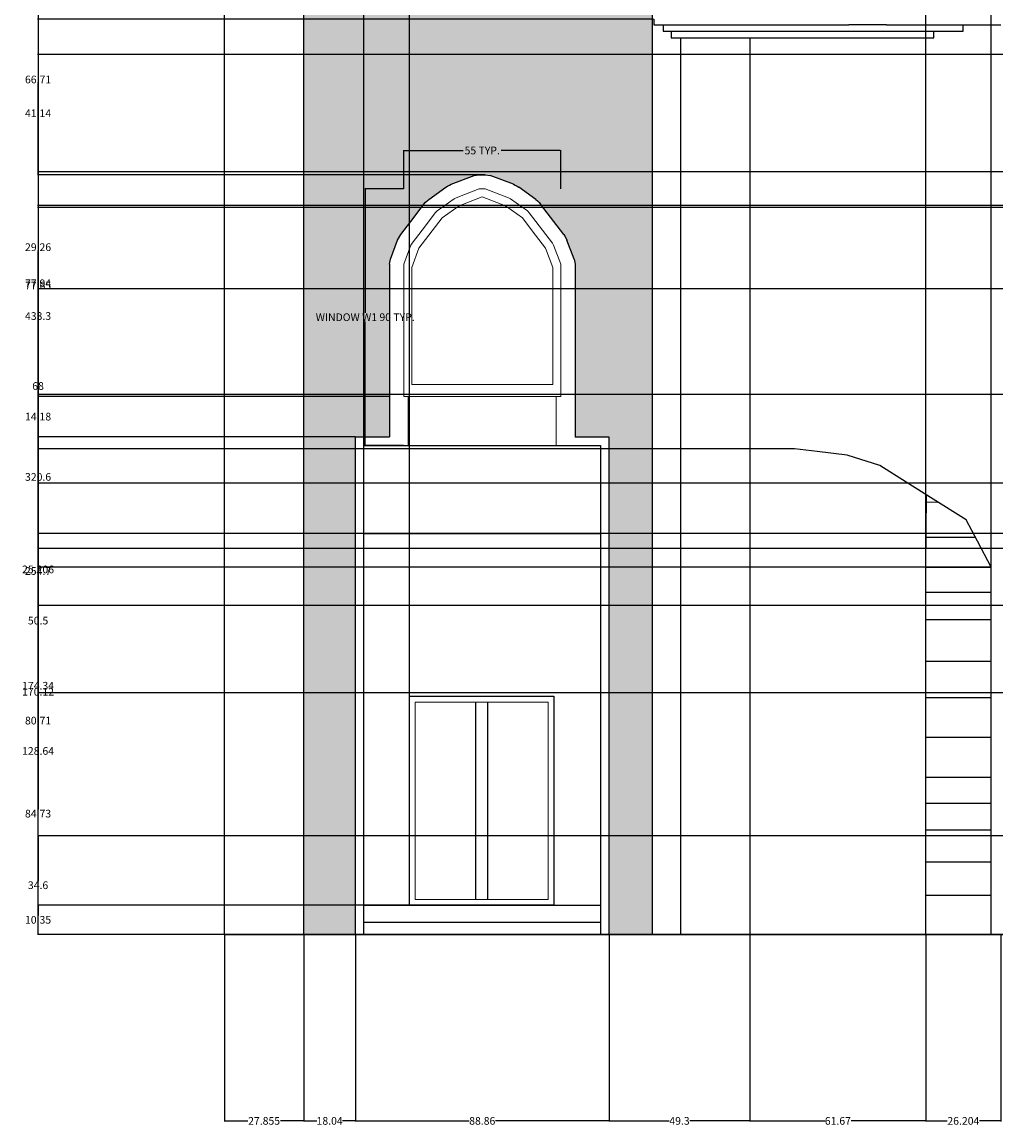
# Model space of a CAD drawing. Units: inches. Extents: x 2 to 1442, y 20 to 729.
# Tile 1 of 8: x 2 to 343, y 20 to 407. Entities that reach past the tile are written whole.
import ezdxf

# ---------------------------------------------------------------- set-up
doc = ezdxf.new("R2010")
doc.units = ezdxf.units.IN
doc.header["$MEASUREMENT"] = 0
for name, color, linetype, lineweight in [('A-ANNO-DIMS', 2, 'Continuous', 18), ('A-DOOR', 3, 'Continuous', 18), ('A-ELEV', 7, 'Continuous', 25), ('A-GLAZ', 4, 'Continuous', 18), ('A-WALL-PATT', 8, 'Continuous', 13)]:
    doc.layers.add(name, color=color, linetype=linetype, lineweight=lineweight)
doc.styles.get("Standard").update_dxf_attribs({"font": 'arial.ttf'})
doc.dimstyles.get("Standard").update_dxf_attribs({"dimtxt": 2.6875, "dimasz": 0.18, "dimexe": 0.18, "dimexo": 0.0625, "dimgap": 0.09, "dimtad": 0, "dimtih": 1, "dimtoh": 1, "dimdec": 4, "dimzin": 0, "dimdsep": 46, "dimlunit": 4, "dimtxsty": 'Standard', "dimcen": 0.09, "dimadec": 0, "dimazin": 0, "dimtfac": 1, "dimtdec": 4, "dimtofl": 0, "dimtmove": 0, "dimatfit": 3, "dimfxl": 1, "dimtolj": 1, "dimtzin": 0, "dimarcsym": 0})

# ---------------------------------------------------------------- blocks, each defined once
blk = doc.blocks.new('WIN-ARCH-TOWER')
for p, q in [((18.34, 86.78), (26.45, 89.83)), ((26.45, 89.83), (28.56, 89.83)), ((36.66, 86.78), (28.56, 89.83)), ((11.69, 82.12), (17.65, 86.41)), ((17.65, 86.41), (18.34, 86.78)), ((19.4, 83.98), (27.5, 87.02)), ((35.6, 83.98), (27.5, 87.02)), ((36.66, 86.78), (37.36, 86.41)), ((43.32, 82.12), (37.36, 86.41)), ((7.58, 76.95), (11.05, 81.5)), ((11.05, 81.5), (11.69, 82.12)), ((13.44, 79.69), (19.4, 83.98)), ((41.56, 79.69), (35.6, 83.98)), ((43.32, 82.12), (43.95, 81.5)), ((47.42, 76.95), (43.95, 81.5)), ((9.97, 75.13), (13.44, 79.69)), ((45.03, 75.13), (41.56, 79.69)), ((2.94, 70.87), (7.58, 76.95)), ((5.33, 69.05), (9.97, 75.13)), ((49.67, 69.05), (45.03, 75.13)), ((52.06, 70.87), (47.42, 76.95)), ((0, 63.44), (2.52, 70.11)), ((2.52, 70.11), (2.94, 70.87)), ((52.06, 70.87), (52.48, 70.11)), ((55, 63.44), (52.48, 70.11)), ((2.81, 62.38), (5.33, 69.05)), ((52.2, 62.38), (49.67, 69.05)), ((0, 63.44), (0, 62.38)), ((0, 62.38), (0, 17.18)), ((2.81, 21.32), (2.81, 62.38)), ((52.2, 21.32), (52.2, 62.38)), ((55, 63.44), (55, 62.38)), ((55, 62.38), (55, 17.41)), ((27.5, 21.32), (2.81, 21.32)), ((24.55, 21.32), (49.24, 21.32)), ((49.24, 21.32), (52.2, 21.32)), ((0, 17.18), (1.6, 17.18)), ((1.6, 0), (1.6, 17.18)), ((1.6, 17.18), (53.4, 17.18)), ((53.4, 0), (53.4, 17.18)), ((53.4, 17.18), (55.01, 17.18)), ((55.01, 17.18), (55, 17.41))]:
    blk.add_line(p, q)
blk = doc.blocks.new('DOOR-DOUBLE')
for points in [[(23.31, 0), (0, 0), (0, 69.12), (23.31, 69.12)], [(23.31, 69.12), (46.63, 69.12), (46.63, 0), (23.31, 0)]]:
    blk.add_lwpolyline(points)
blk = doc.blocks.new('*D5')
at = {"layer": 'A-ANNO-DIMS', "color": 0, "lineweight": -2, "transparency": 16777216}
for p, q in [((135.28, 348.44), (121.69, 348.44)), ((121.87, 348.26), (121.87, 305.01)), ((121.87, 258.79), (121.87, 302.05)), ((135.28, 258.61), (121.69, 258.61))]:
    blk.add_line(p, q, dxfattribs=at)
at = {"layer": 'A-ANNO-DIMS', "color": 0, "transparency": 16777216}
for points in [[(121.84, 348.26), (121.9, 348.26), (121.87, 348.44)], [(121.84, 258.79), (121.9, 258.79), (121.87, 258.61)]]:
    blk.add_solid(points, dxfattribs=at)
at = {"layer": 'Defpoints', "color": 0, "transparency": 16777216}
for p in [(121.87, 348.44), (135.35, 348.44), (135.35, 258.61)]:
    blk.add_point(p, dxfattribs=at)
at = {"layer": 'A-ANNO-DIMS', "color": 0, "transparency": 16777216, "insert": (121.87, 303.53), "char_height": 2.6875, "attachment_point": 5}
blk.add_mtext('\\A1;WINDOW W1 90 TYP.', dxfattribs=at)
blk = doc.blocks.new('*D6')
at = {"layer": 'A-ANNO-DIMS', "color": 0, "lineweight": -2, "transparency": 16777216}
for p, q in [((135.35, 348.5), (135.35, 362.09)), ((135.53, 361.91), (156.22, 361.91)), ((190.17, 361.91), (169.48, 361.91)), ((190.35, 348.5), (190.35, 362.09))]:
    blk.add_line(p, q, dxfattribs=at)
at = {"layer": 'A-ANNO-DIMS', "color": 0, "transparency": 16777216}
for points in [[(135.53, 361.94), (135.53, 361.88), (135.35, 361.91)], [(190.17, 361.94), (190.17, 361.88), (190.35, 361.91)]]:
    blk.add_solid(points, dxfattribs=at)
at = {"layer": 'Defpoints', "color": 0, "transparency": 16777216}
for p in [(190.35, 361.91), (135.35, 348.44), (190.35, 348.44)]:
    blk.add_point(p, dxfattribs=at)
at = {"layer": 'A-ANNO-DIMS', "color": 0, "transparency": 16777216, "insert": (162.85, 361.91), "char_height": 2.6875, "attachment_point": 5}
blk.add_mtext('\\A1;55 TYP.', dxfattribs=at)
blk = doc.blocks.new('*D13')
at = {"layer": 'A-ANNO-DIMS', "color": 0, "lineweight": -2, "transparency": 16777216}
for p, q in [((72.53, 87.21), (72.53, 21.84)), ((100.38, 87.21), (100.38, 21.84)), ((72.71, 22.02), (80.75, 22.02)), ((100.2, 22.02), (92.16, 22.02))]:
    blk.add_line(p, q, dxfattribs=at)
at = {"layer": 'A-ANNO-DIMS', "color": 0, "transparency": 16777216}
for points in [[(72.71, 22.05), (72.71, 21.99), (72.53, 22.02)], [(100.2, 22.05), (100.2, 21.99), (100.38, 22.02)]]:
    blk.add_solid(points, dxfattribs=at)
at = {"layer": 'Defpoints', "color": 0, "transparency": 16777216}
for p in [(72.53, 87.27), (100.38, 87.27), (100.38, 22.02)]:
    blk.add_point(p, dxfattribs=at)
at = {"layer": 'A-ANNO-DIMS', "color": 0, "transparency": 16777216, "insert": (86.45, 22.02), "char_height": 2.688, "attachment_point": 5}
blk.add_mtext('\\A1;27.855', dxfattribs=at)
blk = doc.blocks.new('*D14')
at = {"layer": 'A-ANNO-DIMS', "color": 0, "lineweight": -2, "transparency": 16777216}
for p, q in [((100.38, 87.21), (100.38, 21.84)), ((118.42, 87.21), (118.42, 21.84)), ((100.56, 22.02), (104.91, 22.02)), ((118.24, 22.02), (113.9, 22.02))]:
    blk.add_line(p, q, dxfattribs=at)
at = {"layer": 'A-ANNO-DIMS', "color": 0, "transparency": 16777216}
for points in [[(100.56, 22.05), (100.56, 21.99), (100.38, 22.02)], [(118.24, 22.05), (118.24, 21.99), (118.42, 22.02)]]:
    blk.add_solid(points, dxfattribs=at)
at = {"layer": 'Defpoints', "color": 0, "transparency": 16777216}
for p in [(100.38, 87.27), (118.42, 87.27), (118.42, 22.02)]:
    blk.add_point(p, dxfattribs=at)
at = {"layer": 'A-ANNO-DIMS', "color": 0, "transparency": 16777216, "insert": (109.4, 22.02), "char_height": 2.688, "attachment_point": 5}
blk.add_mtext('\\A1;18.04', dxfattribs=at)
blk = doc.blocks.new('*D15')
at = {"layer": 'A-ANNO-DIMS', "color": 0, "lineweight": -2, "transparency": 16777216}
for p, q in [((118.42, 87.21), (118.42, 21.84)), ((207.28, 87.21), (207.28, 21.84)), ((118.6, 22.02), (158.23, 22.02)), ((207.1, 22.02), (167.48, 22.02))]:
    blk.add_line(p, q, dxfattribs=at)
at = {"layer": 'A-ANNO-DIMS', "color": 0, "transparency": 16777216}
for points in [[(118.6, 22.05), (118.6, 21.99), (118.42, 22.02)], [(207.1, 22.05), (207.1, 21.99), (207.28, 22.02)]]:
    blk.add_solid(points, dxfattribs=at)
at = {"layer": 'Defpoints', "color": 0, "transparency": 16777216}
for p in [(118.42, 87.27), (207.28, 87.27), (207.28, 22.02)]:
    blk.add_point(p, dxfattribs=at)
at = {"layer": 'A-ANNO-DIMS', "color": 0, "transparency": 16777216, "insert": (162.85, 22.02), "char_height": 2.688, "attachment_point": 5}
blk.add_mtext('\\A1;88.86', dxfattribs=at)
blk = doc.blocks.new('*D16')
at = {"layer": 'A-ANNO-DIMS', "color": 0, "lineweight": -2, "transparency": 16777216}
for p, q in [((207.28, 87.21), (207.28, 21.84)), ((256.58, 87.21), (256.58, 21.84)), ((207.46, 22.02), (228.29, 22.02)), ((256.4, 22.02), (235.56, 22.02))]:
    blk.add_line(p, q, dxfattribs=at)
at = {"layer": 'A-ANNO-DIMS', "color": 0, "transparency": 16777216}
for points in [[(207.46, 22.05), (207.46, 21.99), (207.28, 22.02)], [(256.4, 22.05), (256.4, 21.99), (256.58, 22.02)]]:
    blk.add_solid(points, dxfattribs=at)
at = {"layer": 'Defpoints', "color": 0, "transparency": 16777216}
for p in [(207.28, 87.27), (256.58, 87.27), (256.58, 22.02)]:
    blk.add_point(p, dxfattribs=at)
at = {"layer": 'A-ANNO-DIMS', "color": 0, "transparency": 16777216, "insert": (231.93, 22.02), "char_height": 2.688, "attachment_point": 5}
blk.add_mtext('\\A1;49.3', dxfattribs=at)
blk = doc.blocks.new('*D17')
at = {"layer": 'A-ANNO-DIMS', "color": 0, "lineweight": -2, "transparency": 16777216}
for p, q in [((256.58, 87.21), (256.58, 21.84)), ((318.25, 87.21), (318.25, 21.84)), ((256.76, 22.02), (282.78, 22.02)), ((318.07, 22.02), (292.04, 22.02))]:
    blk.add_line(p, q, dxfattribs=at)
at = {"layer": 'A-ANNO-DIMS', "color": 0, "transparency": 16777216}
for points in [[(256.76, 22.05), (256.76, 21.99), (256.58, 22.02)], [(318.07, 22.05), (318.07, 21.99), (318.25, 22.02)]]:
    blk.add_solid(points, dxfattribs=at)
at = {"layer": 'Defpoints', "color": 0, "transparency": 16777216}
for p in [(256.58, 87.27), (318.25, 87.27), (318.25, 22.02)]:
    blk.add_point(p, dxfattribs=at)
at = {"layer": 'A-ANNO-DIMS', "color": 0, "transparency": 16777216, "insert": (287.41, 22.02), "char_height": 2.688, "attachment_point": 5}
blk.add_mtext('\\A1;61.67', dxfattribs=at)
blk = doc.blocks.new('*D18')
at = {"layer": 'A-ANNO-DIMS', "color": 0, "lineweight": -2, "transparency": 16777216}
for p, q in [((318.25, 87.21), (318.25, 21.84)), ((344.45, 87.21), (344.45, 21.84)), ((318.43, 22.02), (325.66, 22.02)), ((344.27, 22.02), (337.04, 22.02))]:
    blk.add_line(p, q, dxfattribs=at)
at = {"layer": 'A-ANNO-DIMS', "color": 0, "transparency": 16777216}
for points in [[(318.43, 22.05), (318.43, 21.99), (318.25, 22.02)], [(344.27, 22.05), (344.27, 21.99), (344.45, 22.02)]]:
    blk.add_solid(points, dxfattribs=at)
at = {"layer": 'Defpoints', "color": 0, "transparency": 16777216}
for p in [(318.25, 87.27), (344.45, 87.27), (344.45, 22.02)]:
    blk.add_point(p, dxfattribs=at)
at = {"layer": 'A-ANNO-DIMS', "color": 0, "transparency": 16777216, "insert": (331.35, 22.02), "char_height": 2.688, "attachment_point": 5}
blk.add_mtext('\\A1;26.204', dxfattribs=at)
blk = doc.blocks.new('*D32')
at = {"layer": 'A-ANNO-DIMS', "color": 0, "lineweight": -2, "transparency": 16777216}
for p, q in [((72.46, 520.58), (7.1, 520.58)), ((7.28, 520.4), (7.28, 305.39)), ((7.28, 87.45), (7.28, 302.46)), ((72.46, 87.27), (7.1, 87.27))]:
    blk.add_line(p, q, dxfattribs=at)
at = {"layer": 'A-ANNO-DIMS', "color": 0, "transparency": 16777216}
for points in [[(7.25, 520.4), (7.31, 520.4), (7.28, 520.58)], [(7.25, 87.45), (7.31, 87.45), (7.28, 87.27)]]:
    blk.add_solid(points, dxfattribs=at)
at = {"layer": 'Defpoints', "color": 0, "transparency": 16777216}
for p in [(7.28, 520.58), (72.53, 520.58), (72.53, 87.27)]:
    blk.add_point(p, dxfattribs=at)
at = {"layer": 'A-ANNO-DIMS', "color": 0, "transparency": 16777216, "insert": (7.28, 303.93), "char_height": 2.688, "attachment_point": 5}
blk.add_mtext('\\A1;433.3', dxfattribs=at)
blk = doc.blocks.new('*D34')
at = {"layer": 'A-ANNO-DIMS', "color": 0, "lineweight": -2, "transparency": 16777216}
for p, q in [((118.36, 261.61), (7.1, 261.61)), ((7.28, 261.43), (7.28, 175.9)), ((7.28, 87.45), (7.28, 172.98)), ((100.32, 87.27), (7.1, 87.27))]:
    blk.add_line(p, q, dxfattribs=at)
at = {"layer": 'A-ANNO-DIMS', "color": 0, "transparency": 16777216}
for points in [[(7.25, 261.43), (7.31, 261.43), (7.28, 261.61)], [(7.25, 87.45), (7.31, 87.45), (7.28, 87.27)]]:
    blk.add_solid(points, dxfattribs=at)
at = {"layer": 'Defpoints', "color": 0, "transparency": 16777216}
for p in [(118.42, 261.61), (7.28, 87.27), (100.38, 87.27)]:
    blk.add_point(p, dxfattribs=at)
at = {"layer": 'A-ANNO-DIMS', "color": 0, "transparency": 16777216, "insert": (7.28, 174.44), "char_height": 2.688, "attachment_point": 5}
blk.add_mtext('\\A1;174.34', dxfattribs=at)
blk = doc.blocks.new('*D35')
at = {"layer": 'A-ANNO-DIMS', "color": 0, "lineweight": -2, "transparency": 16777216}
for p, q in [((130.28, 275.79), (7.1, 275.79)), ((7.28, 275.61), (7.28, 270.16)), ((7.28, 261.79), (7.28, 267.24)), ((118.36, 261.61), (7.1, 261.61))]:
    blk.add_line(p, q, dxfattribs=at)
at = {"layer": 'A-ANNO-DIMS', "color": 0, "transparency": 16777216}
for points in [[(7.25, 275.61), (7.31, 275.61), (7.28, 275.79)], [(7.25, 261.79), (7.31, 261.79), (7.28, 261.61)]]:
    blk.add_solid(points, dxfattribs=at)
at = {"layer": 'Defpoints', "color": 0, "transparency": 16777216}
for p in [(7.28, 275.79), (130.35, 275.79), (118.42, 261.61)]:
    blk.add_point(p, dxfattribs=at)
at = {"layer": 'A-ANNO-DIMS', "color": 0, "transparency": 16777216, "insert": (7.28, 268.7), "char_height": 2.688, "attachment_point": 5}
blk.add_mtext('\\A1;14.18', dxfattribs=at)
blk = doc.blocks.new('*D36')
at = {"layer": 'A-ANNO-DIMS', "color": 0, "lineweight": -2, "transparency": 16777216}
for p, q in [((163.84, 353.44), (7.1, 353.44)), ((7.28, 353.26), (7.28, 316.08)), ((7.28, 275.97), (7.28, 313.15)), ((130.28, 275.79), (7.1, 275.79))]:
    blk.add_line(p, q, dxfattribs=at)
at = {"layer": 'A-ANNO-DIMS', "color": 0, "transparency": 16777216}
for points in [[(7.25, 353.26), (7.31, 353.26), (7.28, 353.44)], [(7.25, 275.97), (7.31, 275.97), (7.28, 275.79)]]:
    blk.add_solid(points, dxfattribs=at)
at = {"layer": 'Defpoints', "color": 0, "transparency": 16777216}
for p in [(7.28, 353.44), (163.9, 353.44), (130.35, 275.79)]:
    blk.add_point(p, dxfattribs=at)
at = {"layer": 'A-ANNO-DIMS', "color": 0, "transparency": 16777216, "insert": (7.28, 314.62), "char_height": 2.688, "attachment_point": 5}
blk.add_mtext('\\A1;77.65', dxfattribs=at)
blk = doc.blocks.new('*D37')
at = {"layer": 'A-ANNO-DIMS', "color": 0, "lineweight": -2, "transparency": 16777216}
for p, q in [((144.79, 420.15), (7.1, 420.15)), ((7.28, 419.97), (7.28, 388.26)), ((7.28, 353.62), (7.28, 385.33)), ((163.84, 353.44), (7.1, 353.44))]:
    blk.add_line(p, q, dxfattribs=at)
at = {"layer": 'A-ANNO-DIMS', "color": 0, "transparency": 16777216}
for points in [[(7.25, 419.97), (7.31, 419.97), (7.28, 420.15)], [(7.25, 353.62), (7.31, 353.62), (7.28, 353.44)]]:
    blk.add_solid(points, dxfattribs=at)
at = {"layer": 'Defpoints', "color": 0, "transparency": 16777216}
for p in [(7.28, 420.15), (144.86, 420.15), (163.9, 353.44)]:
    blk.add_point(p, dxfattribs=at)
at = {"layer": 'A-ANNO-DIMS', "color": 0, "transparency": 16777216, "insert": (7.28, 386.79), "char_height": 2.688, "attachment_point": 5}
blk.add_mtext('\\A1;66.71', dxfattribs=at)
blk = doc.blocks.new('*D41')
at = {"layer": 'A-ANNO-DIMS', "color": 0, "lineweight": -2, "transparency": 16777216}
for p, q in [((137.28, 97.62), (7.1, 97.62)), ((7.28, 97.44), (7.28, 93.91)), ((7.28, 87.45), (7.28, 90.98)), ((121.36, 87.27), (7.1, 87.27))]:
    blk.add_line(p, q, dxfattribs=at)
at = {"layer": 'A-ANNO-DIMS', "color": 0, "transparency": 16777216}
for points in [[(7.25, 97.44), (7.31, 97.44), (7.28, 97.62)], [(7.25, 87.45), (7.31, 87.45), (7.28, 87.27)]]:
    blk.add_solid(points, dxfattribs=at)
at = {"layer": 'Defpoints', "color": 0, "transparency": 16777216}
for p in [(137.34, 97.62), (7.28, 87.27), (121.42, 87.27)]:
    blk.add_point(p, dxfattribs=at)
at = {"layer": 'A-ANNO-DIMS', "color": 0, "transparency": 16777216, "insert": (7.28, 92.45), "char_height": 2.688, "attachment_point": 5}
blk.add_mtext('\\A1;10.35', dxfattribs=at)
blk = doc.blocks.new('*D42')
at = {"layer": 'A-ANNO-DIMS', "color": 0, "lineweight": -2, "transparency": 16777216}
for p, q in [((121.42, 97.68), (121.42, 726.93)), ((137.34, 97.68), (137.34, 726.93)), ((121.6, 726.75), (123.84, 726.75)), ((137.16, 726.75), (134.93, 726.75))]:
    blk.add_line(p, q, dxfattribs=at)
at = {"layer": 'A-ANNO-DIMS', "color": 0, "transparency": 16777216}
for points in [[(121.6, 726.78), (121.6, 726.72), (121.42, 726.75)], [(137.16, 726.78), (137.16, 726.72), (137.34, 726.75)]]:
    blk.add_solid(points, dxfattribs=at)
at = {"layer": 'Defpoints', "color": 0, "transparency": 16777216}
for p in [(137.34, 726.75), (121.42, 97.62), (137.34, 97.62)]:
    blk.add_point(p, dxfattribs=at)
at = {"layer": 'A-ANNO-DIMS', "color": 0, "transparency": 16777216, "insert": (129.38, 726.75), "char_height": 2.688, "attachment_point": 5}
blk.add_mtext('\\A1;15.918', dxfattribs=at)
blk = doc.blocks.new('*D43')
at = {"layer": 'A-ANNO-DIMS', "color": 0, "lineweight": -2, "transparency": 16777216}
for p, q in [((222.84, 407.89), (7.1, 407.89)), ((7.28, 407.71), (7.28, 249.04)), ((7.28, 87.45), (7.28, 246.12)), ((232.22, 87.27), (7.1, 87.27))]:
    blk.add_line(p, q, dxfattribs=at)
at = {"layer": 'A-ANNO-DIMS', "color": 0, "transparency": 16777216}
for points in [[(7.25, 407.71), (7.31, 407.71), (7.28, 407.89)], [(7.25, 87.45), (7.31, 87.45), (7.28, 87.27)]]:
    blk.add_solid(points, dxfattribs=at)
at = {"layer": 'Defpoints', "color": 0, "transparency": 16777216}
for p in [(7.28, 407.89), (222.9, 407.89), (232.28, 87.27)]:
    blk.add_point(p, dxfattribs=at)
at = {"layer": 'A-ANNO-DIMS', "color": 0, "transparency": 16777216, "insert": (7.28, 247.58), "char_height": 2.688, "attachment_point": 5}
blk.add_mtext('\\A1;320.6', dxfattribs=at)
blk = doc.blocks.new('*D46')
at = {"layer": 'A-ANNO-DIMS', "color": 0, "lineweight": -2, "transparency": 16777216}
for p, q in [((341, 215.92), (7.1, 215.92)), ((7.28, 215.74), (7.28, 153.06)), ((7.28, 87.45), (7.28, 150.13)), ((318.18, 87.27), (7.1, 87.27))]:
    blk.add_line(p, q, dxfattribs=at)
at = {"layer": 'A-ANNO-DIMS', "color": 0, "transparency": 16777216}
for points in [[(7.25, 215.74), (7.31, 215.74), (7.28, 215.92)], [(7.25, 87.45), (7.31, 87.45), (7.28, 87.27)]]:
    blk.add_solid(points, dxfattribs=at)
at = {"layer": 'Defpoints', "color": 0, "transparency": 16777216}
for p in [(7.28, 215.92), (341.06, 215.92), (318.25, 87.27)]:
    blk.add_point(p, dxfattribs=at)
at = {"layer": 'A-ANNO-DIMS', "color": 0, "transparency": 16777216, "insert": (7.28, 151.59), "char_height": 2.688, "attachment_point": 5}
blk.add_mtext('\\A1;128.64', dxfattribs=at)
blk = doc.blocks.new('*D47')
at = {"layer": 'A-ANNO-DIMS', "color": 0, "lineweight": -2, "transparency": 16777216}
for p, q in [((318.25, 215.98), (318.25, 726.93)), ((341.06, 215.98), (341.06, 726.93)), ((318.43, 726.75), (323.95, 726.75)), ((340.88, 726.75), (335.36, 726.75))]:
    blk.add_line(p, q, dxfattribs=at)
at = {"layer": 'A-ANNO-DIMS', "color": 0, "transparency": 16777216}
for points in [[(318.43, 726.78), (318.43, 726.72), (318.25, 726.75)], [(340.88, 726.78), (340.88, 726.72), (341.06, 726.75)]]:
    blk.add_solid(points, dxfattribs=at)
at = {"layer": 'Defpoints', "color": 0, "transparency": 16777216}
for p in [(341.06, 726.75), (318.25, 215.92), (341.06, 215.92)]:
    blk.add_point(p, dxfattribs=at)
at = {"layer": 'A-ANNO-DIMS', "color": 0, "transparency": 16777216, "insert": (329.65, 726.75), "char_height": 2.688, "attachment_point": 5}
blk.add_mtext('\\A1;22.815', dxfattribs=at)
blk = doc.blocks.new('*D48')
at = {"layer": 'A-ANNO-DIMS', "color": 0, "lineweight": -2, "transparency": 16777216}
for p, q in [((256.51, 257.39), (7.1, 257.39)), ((7.28, 257.21), (7.28, 173.79)), ((7.28, 87.45), (7.28, 170.87)), ((256.51, 87.27), (7.1, 87.27))]:
    blk.add_line(p, q, dxfattribs=at)
at = {"layer": 'A-ANNO-DIMS', "color": 0, "transparency": 16777216}
for points in [[(7.25, 257.21), (7.31, 257.21), (7.28, 257.39)], [(7.25, 87.45), (7.31, 87.45), (7.28, 87.27)]]:
    blk.add_solid(points, dxfattribs=at)
at = {"layer": 'Defpoints', "color": 0, "transparency": 16777216}
for p in [(256.58, 257.39), (7.28, 87.27), (256.58, 87.27)]:
    blk.add_point(p, dxfattribs=at)
at = {"layer": 'A-ANNO-DIMS', "color": 0, "transparency": 16777216, "insert": (7.28, 172.33), "char_height": 2.688, "attachment_point": 5}
blk.add_mtext('\\A1;170.12', dxfattribs=at)
blk = doc.blocks.new('*D54')
at = {"layer": 'A-ANNO-DIMS', "color": 0, "lineweight": -2, "transparency": 16777216}
for p, q in [((388.65, 354.39), (7.1, 354.39)), ((7.28, 354.21), (7.28, 316.88)), ((7.28, 276.62), (7.28, 313.95)), ((353.03, 276.44), (7.1, 276.44))]:
    blk.add_line(p, q, dxfattribs=at)
at = {"layer": 'A-ANNO-DIMS', "color": 0, "transparency": 16777216}
for points in [[(7.25, 354.21), (7.31, 354.21), (7.28, 354.39)], [(7.25, 276.62), (7.31, 276.62), (7.28, 276.44)]]:
    blk.add_solid(points, dxfattribs=at)
at = {"layer": 'Defpoints', "color": 0, "transparency": 16777216}
for p in [(7.28, 354.39), (388.71, 354.39), (353.09, 276.44)]:
    blk.add_point(p, dxfattribs=at)
at = {"layer": 'A-ANNO-DIMS', "color": 0, "transparency": 16777216, "insert": (7.28, 315.41), "char_height": 2.688, "attachment_point": 5}
blk.add_mtext('\\A1;77.94', dxfattribs=at)
blk = doc.blocks.new('*D57')
at = {"layer": 'A-ANNO-DIMS', "color": 0, "lineweight": -2, "transparency": 16777216}
for p, q in [((381.96, 395.53), (7.1, 395.53)), ((7.28, 395.35), (7.28, 376.4)), ((7.28, 354.57), (7.28, 373.52)), ((388.65, 354.39), (7.1, 354.39))]:
    blk.add_line(p, q, dxfattribs=at)
at = {"layer": 'A-ANNO-DIMS', "color": 0, "transparency": 16777216}
for points in [[(7.25, 395.35), (7.31, 395.35), (7.28, 395.53)], [(7.25, 354.57), (7.31, 354.57), (7.28, 354.39)]]:
    blk.add_solid(points, dxfattribs=at)
at = {"layer": 'Defpoints', "color": 0, "transparency": 16777216}
for p in [(382.02, 395.53), (7.28, 354.39), (388.71, 354.39)]:
    blk.add_point(p, dxfattribs=at)
at = {"layer": 'A-ANNO-DIMS', "color": 0, "transparency": 16777216, "insert": (7.28, 374.96), "char_height": 2.688, "attachment_point": 5}
blk.add_mtext('\\A1;41.14', dxfattribs=at)
blk = doc.blocks.new('*D72')
at = {"layer": 'A-ANNO-DIMS', "color": 0, "lineweight": -2, "transparency": 16777216}
for p, q in [((585.94, 341.99), (7.1, 341.99)), ((7.28, 341.81), (7.28, 216.09)), ((7.28, 87.45), (7.28, 213.17)), ((592.44, 87.27), (7.1, 87.27))]:
    blk.add_line(p, q, dxfattribs=at)
at = {"layer": 'A-ANNO-DIMS', "color": 0, "transparency": 16777216}
for points in [[(7.25, 341.81), (7.31, 341.81), (7.28, 341.99)], [(7.25, 87.45), (7.31, 87.45), (7.28, 87.27)]]:
    blk.add_solid(points, dxfattribs=at)
at = {"layer": 'Defpoints', "color": 0, "transparency": 16777216}
for p in [(7.28, 341.99), (586, 341.99), (592.5, 87.27)]:
    blk.add_point(p, dxfattribs=at)
at = {"layer": 'A-ANNO-DIMS', "color": 0, "transparency": 16777216, "insert": (7.28, 214.63), "char_height": 2.688, "attachment_point": 5}
blk.add_mtext('\\A1;254.7', dxfattribs=at)
blk = doc.blocks.new('*D74')
at = {"layer": 'A-ANNO-DIMS', "color": 0, "lineweight": -2, "transparency": 16777216}
for p, q in [((655.94, 172), (7.1, 172)), ((7.28, 171.82), (7.28, 131.1)), ((7.28, 87.45), (7.28, 128.17)), ((655.94, 87.27), (7.1, 87.27))]:
    blk.add_line(p, q, dxfattribs=at)
at = {"layer": 'A-ANNO-DIMS', "color": 0, "transparency": 16777216}
for points in [[(7.25, 171.82), (7.31, 171.82), (7.28, 172)], [(7.25, 87.45), (7.31, 87.45), (7.28, 87.27)]]:
    blk.add_solid(points, dxfattribs=at)
at = {"layer": 'Defpoints', "color": 0, "transparency": 16777216}
for p in [(656, 172), (7.28, 87.27), (656, 87.27)]:
    blk.add_point(p, dxfattribs=at)
at = {"layer": 'A-ANNO-DIMS', "color": 0, "transparency": 16777216, "insert": (7.28, 129.64), "char_height": 2.688, "attachment_point": 5}
blk.add_mtext('\\A1;84.73', dxfattribs=at)
blk = doc.blocks.new('*D75')
at = {"layer": 'A-ANNO-DIMS', "color": 0, "lineweight": -2, "transparency": 16777216}
for p, q in [((721.76, 222.5), (7.1, 222.5)), ((7.28, 222.32), (7.28, 198.71)), ((7.28, 172.18), (7.28, 195.79)), ((655.94, 172), (7.1, 172))]:
    blk.add_line(p, q, dxfattribs=at)
at = {"layer": 'A-ANNO-DIMS', "color": 0, "transparency": 16777216}
for points in [[(7.25, 222.32), (7.31, 222.32), (7.28, 222.5)], [(7.25, 172.18), (7.31, 172.18), (7.28, 172)]]:
    blk.add_solid(points, dxfattribs=at)
at = {"layer": 'Defpoints', "color": 0, "transparency": 16777216}
for p in [(7.28, 222.5), (721.83, 222.5), (656, 172)]:
    blk.add_point(p, dxfattribs=at)
at = {"layer": 'A-ANNO-DIMS', "color": 0, "transparency": 16777216, "insert": (7.28, 197.25), "char_height": 2.688, "attachment_point": 5}
blk.add_mtext('\\A1;50.5', dxfattribs=at)
blk = doc.blocks.new('*D76')
at = {"layer": 'A-ANNO-DIMS', "color": 0, "lineweight": -2, "transparency": 16777216}
for p, q in [((470.75, 121.87), (7.1, 121.87)), ((7.28, 121.69), (7.28, 106.03)), ((7.28, 87.45), (7.28, 103.11)), ((470.75, 87.27), (7.1, 87.27))]:
    blk.add_line(p, q, dxfattribs=at)
at = {"layer": 'A-ANNO-DIMS', "color": 0, "transparency": 16777216}
for points in [[(7.25, 121.69), (7.31, 121.69), (7.28, 121.87)], [(7.25, 87.45), (7.31, 87.45), (7.28, 87.27)]]:
    blk.add_solid(points, dxfattribs=at)
at = {"layer": 'Defpoints', "color": 0, "transparency": 16777216}
for p in [(470.81, 121.87), (7.28, 87.27), (470.81, 87.27)]:
    blk.add_point(p, dxfattribs=at)
at = {"layer": 'A-ANNO-DIMS', "color": 0, "transparency": 16777216, "insert": (7.28, 104.57), "char_height": 2.688, "attachment_point": 5}
blk.add_mtext('\\A1;34.6', dxfattribs=at)
blk = doc.blocks.new('*D77')
at = {"layer": 'A-ANNO-DIMS', "color": 0, "lineweight": -2, "transparency": 16777216}
for p, q in [((470.75, 202.58), (7.1, 202.58)), ((7.28, 202.4), (7.28, 163.69)), ((7.28, 122.05), (7.28, 160.77)), ((470.75, 121.87), (7.1, 121.87))]:
    blk.add_line(p, q, dxfattribs=at)
at = {"layer": 'A-ANNO-DIMS', "color": 0, "transparency": 16777216}
for points in [[(7.25, 202.4), (7.31, 202.4), (7.28, 202.58)], [(7.25, 122.05), (7.31, 122.05), (7.28, 121.87)]]:
    blk.add_solid(points, dxfattribs=at)
at = {"layer": 'Defpoints', "color": 0, "transparency": 16777216}
for p in [(7.28, 202.58), (470.81, 202.58), (470.81, 121.87)]:
    blk.add_point(p, dxfattribs=at)
at = {"layer": 'A-ANNO-DIMS', "color": 0, "transparency": 16777216, "insert": (7.28, 162.23), "char_height": 2.688, "attachment_point": 5}
blk.add_mtext('\\A1;80.71', dxfattribs=at)
blk = doc.blocks.new('*D78')
at = {"layer": 'A-ANNO-DIMS', "color": 0, "lineweight": -2, "transparency": 16777216}
for p, q in [((470.75, 227.79), (7.1, 227.79)), ((7.28, 227.61), (7.28, 216.65)), ((7.28, 202.76), (7.28, 213.72)), ((470.75, 202.58), (7.1, 202.58))]:
    blk.add_line(p, q, dxfattribs=at)
at = {"layer": 'A-ANNO-DIMS', "color": 0, "transparency": 16777216}
for points in [[(7.25, 227.61), (7.31, 227.61), (7.28, 227.79)], [(7.25, 202.76), (7.31, 202.76), (7.28, 202.58)]]:
    blk.add_solid(points, dxfattribs=at)
at = {"layer": 'Defpoints', "color": 0, "transparency": 16777216}
for p in [(7.28, 227.79), (470.81, 227.79), (470.81, 202.58)]:
    blk.add_point(p, dxfattribs=at)
at = {"layer": 'A-ANNO-DIMS', "color": 0, "transparency": 16777216, "insert": (7.28, 215.19), "char_height": 2.688, "attachment_point": 5}
blk.add_mtext('\\A1;25.206', dxfattribs=at)
blk = doc.blocks.new('*D79')
at = {"layer": 'A-ANNO-DIMS', "color": 0, "lineweight": -2, "transparency": 16777216}
for p, q in [((489.71, 313.43), (7.1, 313.43)), ((7.28, 313.25), (7.28, 280.88)), ((7.28, 245.6), (7.28, 277.96)), ((489.71, 245.42), (7.1, 245.42))]:
    blk.add_line(p, q, dxfattribs=at)
at = {"layer": 'A-ANNO-DIMS', "color": 0, "transparency": 16777216}
for points in [[(7.25, 313.25), (7.31, 313.25), (7.28, 313.43)], [(7.25, 245.6), (7.31, 245.6), (7.28, 245.42)]]:
    blk.add_solid(points, dxfattribs=at)
at = {"layer": 'Defpoints', "color": 0, "transparency": 16777216}
for p in [(7.28, 313.43), (489.77, 313.43), (489.77, 245.42)]:
    blk.add_point(p, dxfattribs=at)
at = {"layer": 'A-ANNO-DIMS', "color": 0, "transparency": 16777216, "insert": (7.28, 279.42), "char_height": 2.688, "attachment_point": 5}
blk.add_mtext('\\A1;68', dxfattribs=at)
blk = doc.blocks.new('*D80')
at = {"layer": 'A-ANNO-DIMS', "color": 0, "lineweight": -2, "transparency": 16777216}
for p, q in [((526.66, 342.68), (7.1, 342.68)), ((7.28, 342.5), (7.28, 329.52)), ((7.28, 313.61), (7.28, 326.59)), ((489.71, 313.43), (7.1, 313.43))]:
    blk.add_line(p, q, dxfattribs=at)
at = {"layer": 'A-ANNO-DIMS', "color": 0, "transparency": 16777216}
for points in [[(7.25, 342.5), (7.31, 342.5), (7.28, 342.68)], [(7.25, 313.61), (7.31, 313.61), (7.28, 313.43)]]:
    blk.add_solid(points, dxfattribs=at)
at = {"layer": 'Defpoints', "color": 0, "transparency": 16777216}
for p in [(7.28, 342.68), (526.72, 342.68), (489.77, 313.43)]:
    blk.add_point(p, dxfattribs=at)
at = {"layer": 'A-ANNO-DIMS', "color": 0, "transparency": 16777216, "insert": (7.28, 328.05), "char_height": 2.688, "attachment_point": 5}
blk.add_mtext('\\A1;29.26', dxfattribs=at)

msp = doc.modelspace()

# ---------------------------------------------------------------- hatches: boundary and pattern name
at = {"layer": 'A-WALL-PATT'}
h = msp.add_hatch(dxfattribs=at)
h.set_pattern_fill('BRASS', color=256, scale=14)
h.paths.add_polyline_path([(222.3553, 494.0357), (100.382, 494.0357), (100.382, 87.2714), (118.4234, 87.2714), (118.4234, 261.6116), (130.3451, 261.6116), (130.3451, 275.7919), (130.3451, 320.992), (130.3451, 322.0535), (130.6686, 323.8227), (133.191, 330.4901), (134.3119, 332.5101), (138.9535, 338.5974), (142.6478, 343.4423), (143.8105, 344.5736), (150.3377, 349.2734), (151.6201, 349.9601), (160.0334, 353.1203), (161.7915, 353.4396), (163.9013, 353.4396), (165.6594, 353.1203), (174.0727, 349.9601), (175.3551, 349.2734), (181.8823, 344.5736), (183.045, 343.4423), (186.7393, 338.5974), (191.601, 332.2216), (192.3734, 330.8295), (195.0242, 323.8227), (195.3477, 322.0535), (195.3477, 320.992), (195.3477, 276.0187), (195.3477, 261.5562), (207.2798, 261.5562), (207.2798, 87.2714), (222.3553, 87.2714)])
h.paths.add_polyline_path([(144.8571, 420.1495), (144.8571, 464.3282), (148.784, 472.9254), (157.7288, 481.8631), (164.2287, 486.0178), (170.7285, 481.8631), (179.6733, 472.9254), (183.6002, 464.3282), (183.6002, 420.1495)], flags=16)
h.paths.add_polyline_path([(146.8571, 422.1495), (146.8571, 463.893), (150.4531, 471.7659), (158.9889, 480.2948), (164.2287, 483.6441), (169.4684, 480.2948), (178.0042, 471.7659), (181.6002, 463.893), (181.6002, 422.1495)], flags=0)

# ---------------------------------------------------------------- linework, layer by layer
at = {"layer": 'A-ELEV'}
for p, q in [((72.5272, 255.2714), (72.5272, 423.2714)), ((222.8994, 407.8873), (222.8994, 405.9114)), ((222.8994, 405.9114), (249.3478, 405.9114)), ((226.1729, 405.9114), (226.1729, 403.6578)), ((226.1729, 403.6578), (249.3478, 403.6578)), ((229.0144, 403.6578), (229.0144, 401.3516)), ((249.3478, 405.9114), (291.2886, 405.9114)), ((249.3478, 403.6578), (299.4874, 403.6578)), ((304.4461, 405.9114), (291.2886, 405.9114)), ((299.4874, 403.6578), (331.3076, 403.6578)), ((304.4461, 405.9114), (335.8829, 405.9114)), ((321.0095, 401.3516), (321.0095, 403.6578)), ((331.3076, 403.6578), (331.3076, 405.9114)), ((335.8829, 405.9114), (335.8829, 405.9114)), ((335.8829, 405.9114), (344.4513, 405.9114)), ((229.0144, 401.3516), (291.0961, 401.3516)), ((232.2824, 401.3516), (232.2824, 87.2714)), ((256.5766, 401.3516), (256.5766, 87.2714)), ((291.0961, 401.3516), (321.0095, 401.3516)), ((151.9303, 350.0767), (160.0334, 353.1203)), ((161.7915, 353.4396), (163.9013, 353.4396)), ((173.7625, 350.0767), (165.6594, 353.1203)), ((144.1106, 344.7897), (150.0687, 349.0797)), ((150.6298, 349.4298), (151.3279, 349.8037)), ((174.3649, 349.8037), (175.063, 349.4298)), ((181.5822, 344.7897), (175.6241, 349.0797)), ((142.9129, 343.7002), (143.5455, 344.3157)), ((182.1473, 344.3157), (182.7799, 343.7002)), ((138.9535, 338.5974), (142.4236, 343.1483)), ((186.7393, 338.5974), (183.2692, 343.1483)), ((134.3119, 332.5101), (138.9535, 338.5974)), ((191.381, 332.5101), (186.7393, 338.5974)), ((130.6686, 323.8227), (133.191, 330.4901)), ((191.777, 331.9043), (192.1973, 331.1468)), ((195.0242, 323.8227), (192.5018, 330.4901)), ((130.3451, 322.0535), (130.3451, 320.992)), ((130.3451, 320.992), (130.3451, 275.7919)), ((195.3477, 322.0535), (195.3477, 320.992)), ((195.3477, 320.992), (195.3477, 276.0187)), ((130.3451, 275.7919), (130.3451, 261.6116)), ((195.3477, 276.0187), (195.3477, 261.5562)), ((118.4234, 87.2714), (118.4234, 261.6116)), ((118.4234, 261.6116), (130.3451, 261.6116)), ((207.2798, 261.5562), (195.3477, 261.5562)), ((207.2798, 87.2714), (207.2798, 261.5562)), ((72.5272, 87.2714), (72.5272, 255.2714)), ((118.4234, 258.6116), (118.4234, 258.6116)), ((318.2474, 215.9163), (318.4426, 241.3024)), ((318.4235, 238.8156), (322.4558, 238.7967)), ((121.4234, 227.7901), (204.2798, 227.7901)), ((318.3285, 226.4671), (335.5715, 226.4671)), ((318.2474, 87.2714), (318.2474, 215.9163)), ((318.2474, 215.9163), (341.0623, 215.9163)), ((318.2474, 207.1602), (341.0623, 207.1602)), ((318.2474, 197.6038), (341.0623, 197.6038)), ((318.2474, 183.0302), (341.0623, 183.0302)), ((318.2474, 170.3214), (341.0623, 170.3214)), ((318.2474, 156.4645), (341.0623, 156.4645)), ((318.2474, 142.3688), (341.0623, 142.3688)), ((318.2474, 133.2901), (341.0623, 133.2901)), ((318.2474, 123.9726), (341.0623, 123.9726)), ((318.2474, 112.7437), (341.0623, 112.7437)), ((318.2474, 101.0371), (341.0623, 101.0371)), ((121.4234, 97.6222), (204.2798, 97.6222)), ((121.4234, 91.6376), (204.2798, 91.6376)), ((72.5272, 87.2714), (721.8257, 87.2714)), ((121.4234, 87.2714), (118.4234, 87.2714)), ((204.2798, 87.2714), (207.2798, 87.2714))]:
    msp.add_line(p, q, dxfattribs=at)
for points in [[(100.382, 494.0357), (222.3553, 494.0357), (222.3553, 87.2714), (100.382, 87.2714)], [(121.4234, 258.6116), (204.2798, 258.6116), (204.2798, 87.2714), (121.4234, 87.2714)]]:
    msp.add_lwpolyline(points, close=True, dxfattribs=at)
for points in [[(160.0334, 353.1203), (161.7915, 353.4396)], [(163.9013, 353.4396), (165.6594, 353.1203)], [(150.0687, 349.0797), (150.6298, 349.4298)], [(151.3279, 349.8037), (151.9303, 350.0767)], [(173.7625, 350.0767), (174.3649, 349.8037)], [(175.063, 349.4298), (175.6241, 349.0797)], [(143.5455, 344.3157), (144.1106, 344.7897)], [(181.5822, 344.7897), (182.1473, 344.3157)], [(142.4236, 343.1483), (142.9129, 343.7002)], [(182.7799, 343.7002), (183.2692, 343.1483)], [(133.191, 330.4901), (134.3119, 332.5101)], [(191.381, 332.5101), (191.777, 331.9043)], [(192.1973, 331.1468), (192.5018, 330.4901)], [(130.3451, 322.0535), (130.6686, 323.8227)], [(195.0242, 323.8227), (195.3477, 322.0535)], [(302.0658, 251.5273), (290.622, 255.1671), (280.101, 256.4358), (272.1694, 257.3923), (265.4987, 257.3923), (256.5766, 257.3923)], [(341.0623, 87.2714), (341.0623, 215.9163), (336.2785, 225.1085), (332.3793, 232.6009), (320.8232, 239.816), (311.3619, 245.7232), (302.0658, 251.5273), (302.0658, 251.5273)], [(164.6555, 97.6222), (164.6555, 97.6222), (137.3412, 97.6222), (137.3412, 170.7392), (164.6555, 170.7392)], [(160.6555, 170.7392), (187.9698, 170.7392), (187.9698, 97.6222), (160.6555, 97.6222)], [(160.6555, 99.6222), (160.6555, 168.7392)], [(164.6555, 168.7392), (164.6555, 99.6222)]]:
    msp.add_lwpolyline(points, dxfattribs=at)

# ---------------------------------------------------------------- block references
at = {"layer": 'A-DOOR'}
msp.add_blockref('DOOR-DOUBLE', (139.341, 99.622), dxfattribs=at)
at = {"layer": 'A-GLAZ'}
msp.add_blockref('WIN-ARCH-TOWER', (135.345, 258.612), dxfattribs=at)

# ---------------------------------------------------------------- dimensions: what is measured, and where the dimension line sits
at = {"layer": 'A-ANNO-DIMS'}
for base, p1, p2, override, picture, middle in [((137.3412, 726.75), (121.4234, 97.6222), (137.3412, 97.6222), {"dimdec": 3, "dimlfac": 1, "dimrnd": 0, "dimzin": 0, "dimdsep": 46, "dimlunit": 2}, '*D42', (129.3823, 726.75)), ((341.0623, 726.75), (318.2474, 215.9163), (341.0623, 215.9163), {"dimdec": 3, "dimlfac": 1, "dimrnd": 0, "dimzin": 0, "dimdsep": 46, "dimlunit": 2}, '*D47', (329.6548, 726.75)), ((100.382, 22.0214), (72.5272, 87.2714), (100.382, 87.2714), {"dimdec": 3, "dimlfac": 1, "dimrnd": 0, "dimzin": 0, "dimdsep": 46, "dimlunit": 2}, '*D13', (86.4546, 22.0214)), ((118.4234, 22.0214), (100.382, 87.2714), (118.4234, 87.2714), {"dimdec": 2, "dimlfac": 1, "dimrnd": 0, "dimzin": 0, "dimdsep": 46, "dimlunit": 2}, '*D14', (109.4027, 22.0214)), ((207.2798, 22.0214), (118.4234, 87.2714), (207.2798, 87.2714), {"dimdec": 2, "dimlfac": 1, "dimrnd": 0, "dimzin": 0, "dimdsep": 46, "dimlunit": 2}, '*D15', (162.8516, 22.0214)), ((256.5766, 22.0214), (207.2798, 87.2714), (256.5766, 87.2714), {"dimdec": 1, "dimlfac": 1, "dimrnd": 0, "dimzin": 0, "dimdsep": 46, "dimlunit": 2}, '*D16', (231.9282, 22.0214)), ((318.2474, 22.0214), (256.5766, 87.2714), (318.2474, 87.2714), {"dimdec": 2, "dimlfac": 1, "dimrnd": 0, "dimzin": 0, "dimdsep": 46, "dimlunit": 2}, '*D17', (287.412, 22.0214)), ((344.4513, 22.0214), (318.2474, 87.2714), (344.4513, 87.2714), {"dimdec": 3, "dimlfac": 1, "dimrnd": 0, "dimzin": 0, "dimdsep": 46, "dimlunit": 2}, '*D18', (331.3493, 22.0214))]:
    dim = msp.add_linear_dim(base=base, p1=p1, p2=p2, dimstyle='Standard', override=override, dxfattribs=at)
    dim.commit()
    dim.dimension.update_dxf_attribs({"geometry": picture, "text_midpoint": middle})
for base, p1, p2, override, picture, middle in [((7.2772, 520.5823), (72.5272, 87.2714), (72.5272, 520.5823), {"dimdec": 1, "dimlfac": 1, "dimrnd": 0, "dimzin": 0, "dimdsep": 46, "dimlunit": 2}, '*D32', (7.2772, 303.9269)), ((7.2772, 420.1495), (163.9013, 353.4396), (144.8571, 420.1495), {"dimdec": 2, "dimlfac": 1, "dimrnd": 0, "dimzin": 0, "dimdsep": 46, "dimlunit": 2}, '*D37', (7.2772, 386.7945)), ((7.2772, 407.8873), (232.2824, 87.2714), (222.8994, 407.8873), {"dimdec": 1, "dimlfac": 1, "dimrnd": 0, "dimzin": 0, "dimdsep": 46, "dimlunit": 2}, '*D43', (7.2772, 247.5793)), ((7.2772, 354.3865), (382.0241, 395.5258), (388.7085, 354.3865), {"dimdec": 2, "dimlfac": 1, "dimrnd": 0, "dimzin": 0, "dimdsep": 46, "dimlunit": 2}, '*D57', (7.2772, 374.9561)), ((7.2772, 354.3865), (353.095, 276.443), (388.7085, 354.3865), {"dimdec": 2, "dimlfac": 1, "dimrnd": 0, "dimzin": 0, "dimdsep": 46, "dimlunit": 2}, '*D54', (7.2772, 315.4147)), ((7.2772, 353.4396), (130.3451, 275.7919), (163.9013, 353.4396), {"dimdec": 2, "dimlfac": 1, "dimrnd": 0, "dimzin": 0, "dimdsep": 46, "dimlunit": 2}, '*D36', (7.2772, 314.6157)), ((7.2772, 342.6839), (489.7727, 313.4256), (526.72, 342.6839), {"dimdec": 2, "dimlfac": 1, "dimrnd": 0, "dimzin": 0, "dimdsep": 46, "dimlunit": 2}, '*D80', (7.2772, 328.0547)), ((7.2772, 341.9894), (592.5, 87.2714), (586, 341.9894), {"dimdec": 1, "dimlfac": 1, "dimrnd": 0, "dimzin": 0, "dimdsep": 46, "dimlunit": 2}, '*D72', (7.2772, 214.6304)), ((7.2772, 313.4256), (489.7727, 245.4201), (489.7727, 313.4256), {"dimdec": 0, "dimlfac": 1, "dimrnd": 0, "dimzin": 0, "dimdsep": 46, "dimlunit": 2}, '*D79', (7.2772, 279.4228)), ((7.2772, 275.7919), (118.4234, 261.6116), (130.3451, 275.7919), {"dimdec": 2, "dimlfac": 1, "dimrnd": 0, "dimzin": 0, "dimdsep": 46, "dimlunit": 2}, '*D35', (7.2772, 268.7017)), ((7.2772, 87.2714), (118.4234, 261.6116), (100.382, 87.2714), {"dimdec": 2, "dimlfac": 1, "dimrnd": 0, "dimzin": 0, "dimdsep": 46, "dimlunit": 2}, '*D34', (7.2772, 174.4415)), ((7.2772, 87.2714), (256.5766, 257.3923), (256.5766, 87.2714), {"dimdec": 2, "dimlfac": 1, "dimrnd": 0, "dimzin": 0, "dimdsep": 46, "dimlunit": 2}, '*D48', (7.2772, 172.3319)), ((7.2772, 227.7901), (470.8143, 202.5842), (470.8143, 227.7901), {"dimdec": 3, "dimlfac": 1, "dimrnd": 0, "dimzin": 0, "dimdsep": 46, "dimlunit": 2}, '*D78', (7.2772, 215.1871)), ((7.2772, 222.5), (656, 172), (721.8257, 222.5), {"dimdec": 1, "dimlfac": 1, "dimrnd": 0, "dimzin": 0, "dimdsep": 46, "dimlunit": 2}, '*D75', (7.2772, 197.25)), ((7.2772, 215.9163), (318.2474, 87.2714), (341.0623, 215.9163), {"dimdec": 2, "dimlfac": 1, "dimrnd": 0, "dimzin": 0, "dimdsep": 46, "dimlunit": 2}, '*D46', (7.2772, 151.5939)), ((7.2772, 202.5842), (470.8143, 121.871), (470.8143, 202.5842), {"dimdec": 2, "dimlfac": 1, "dimrnd": 0, "dimzin": 0, "dimdsep": 46, "dimlunit": 2}, '*D77', (7.2772, 162.2276)), ((7.2772, 87.2714), (656, 172), (656, 87.2714), {"dimdec": 2, "dimlfac": 1, "dimrnd": 0, "dimzin": 0, "dimdsep": 46, "dimlunit": 2}, '*D74', (7.2772, 129.6357)), ((7.2772, 87.2714), (470.8143, 121.871), (470.8143, 87.2714), {"dimdec": 1, "dimlfac": 1, "dimrnd": 0, "dimzin": 0, "dimdsep": 46, "dimlunit": 2}, '*D76', (7.2772, 104.5712)), ((7.2772, 87.2714), (137.3412, 97.6222), (121.4234, 87.2714), {"dimdec": 2, "dimlfac": 1, "dimrnd": 0, "dimzin": 0, "dimdsep": 46, "dimlunit": 2}, '*D41', (7.2772, 92.4468))]:
    dim = msp.add_linear_dim(base=base, p1=p1, p2=p2, angle=90, dimstyle='Standard', override=override, dxfattribs=at)
    dim.commit()
    dim.dimension.update_dxf_attribs({"geometry": picture, "text_midpoint": middle})
dim = msp.add_linear_dim(base=(190.3508, 361.9138), p1=(135.3451, 348.4396), p2=(190.3508, 348.4396), text='<> TYP.', dimstyle='Standard', override={"dimdec": 0, "dimrnd": 0, "dimzin": 0, "dimlunit": 2}, dxfattribs=at)
dim.commit()
dim.dimension.update_dxf_attribs({"geometry": '*D6', "text_midpoint": (162.848, 361.9138)})
dim = msp.add_linear_dim(base=(121.8709, 348.4396), p1=(135.3451, 258.6116), p2=(135.3451, 348.4396), angle=90, text='WINDOW W1 <> TYP.', dimstyle='Standard', override={"dimdec": 0, "dimrnd": 0, "dimzin": 0, "dimlunit": 2}, dxfattribs=at)
dim.commit()
dim.dimension.update_dxf_attribs({"geometry": '*D5', "text_midpoint": (121.8709, 303.5256)})

doc.saveas('drawing.dxf')
